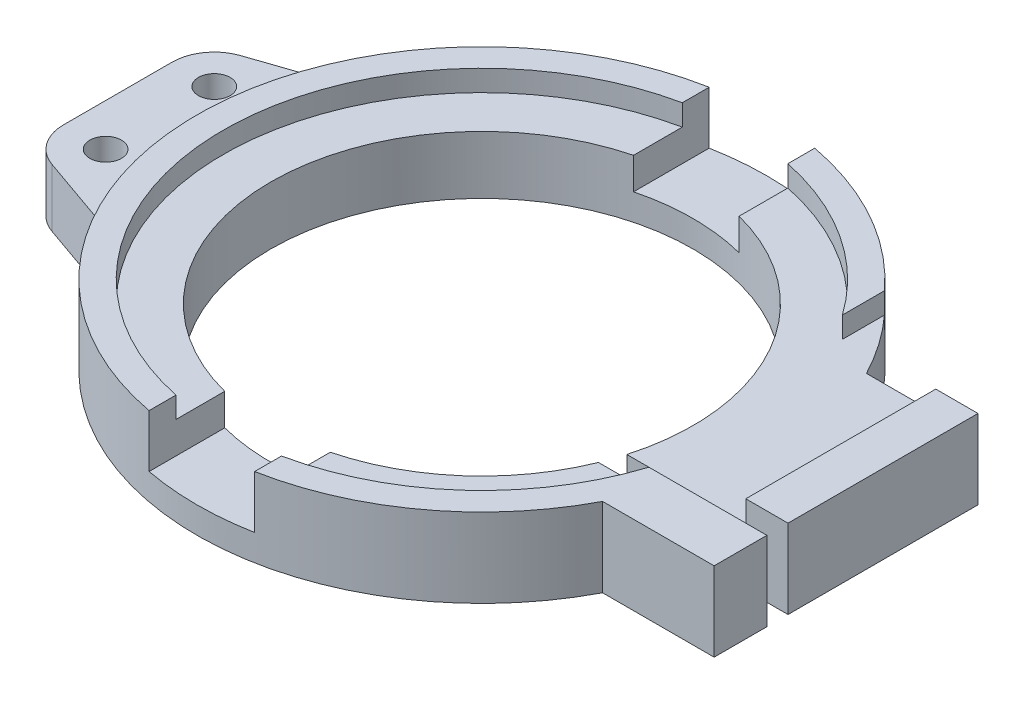
ISO-10303-21;
HEADER;
FILE_DESCRIPTION(('STEP AP214'),'2;1');
FILE_NAME('part.step','',(''),(''),'','','');
FILE_SCHEMA(('AUTOMOTIVE_DESIGN { 1 0 10303 214 1 1 1 1 }'));
ENDSEC;
DATA;
#1=APPLICATION_CONTEXT('core data for automotive mechanical design processes');
#2=APPLICATION_PROTOCOL_DEFINITION('international standard','automotive_design',2000,#1);
#3=PRODUCT_CONTEXT('',#1,'mechanical');
#4=PRODUCT('Part','Part','',(#3));
#5=PRODUCT_RELATED_PRODUCT_CATEGORY('part','',(#4));
#6=PRODUCT_DEFINITION_FORMATION('','',#4);
#7=PRODUCT_DEFINITION_CONTEXT('part definition',#1,'design');
#8=PRODUCT_DEFINITION('design','',#6,#7);
#9=PRODUCT_DEFINITION_SHAPE('','',#8);
#10=(LENGTH_UNIT() NAMED_UNIT(*) SI_UNIT(.MILLI.,.METRE.));
#11=(NAMED_UNIT(*) PLANE_ANGLE_UNIT() SI_UNIT($,.RADIAN.));
#12=(NAMED_UNIT(*) SI_UNIT($,.STERADIAN.) SOLID_ANGLE_UNIT());
#13=UNCERTAINTY_MEASURE_WITH_UNIT(LENGTH_MEASURE(1.E-05),#10,'distance_accuracy_value','');
#14=(GEOMETRIC_REPRESENTATION_CONTEXT(3) GLOBAL_UNCERTAINTY_ASSIGNED_CONTEXT((#13)) GLOBAL_UNIT_ASSIGNED_CONTEXT((#10,
#11,#12)) REPRESENTATION_CONTEXT('',''));
#15=CARTESIAN_POINT('',(0.,0.,0.));
#16=DIRECTION('',(0.,0.,1.));
#17=DIRECTION('',(1.,0.,0.));
#18=AXIS2_PLACEMENT_3D('',#15,#16,#17);
#19=CARTESIAN_POINT('',(0.,15.,0.));
#20=DIRECTION('',(0.,-1.,0.));
#21=DIRECTION('',(0.,0.,-1.));
#22=AXIS2_PLACEMENT_3D('',#19,#20,#21);
#23=CYLINDRICAL_SURFACE('',#22,54.);
#24=DIRECTION('',(0.,-1.,0.));
#25=VECTOR('',#24,1.);
#26=CARTESIAN_POINT('',(47.8643917750973,11.,-25.));
#27=LINE('',#26,#25);
#28=CARTESIAN_POINT('',(47.8643917750973,11.,-25.));
#29=VERTEX_POINT('',#28);
#30=CARTESIAN_POINT('',(47.8643917750973,0.,-25.));
#31=VERTEX_POINT('',#30);
#32=EDGE_CURVE('E58',#29,#31,#27,.T.);
#33=ORIENTED_EDGE('',*,*,#32,.T.);
#34=CARTESIAN_POINT('',(0.,0.,0.));
#35=DIRECTION('',(0.,1.,0.));
#36=DIRECTION('',(0.,0.,1.));
#37=AXIS2_PLACEMENT_3D('',#34,#35,#36);
#38=CIRCLE('',#37,54.);
#39=CARTESIAN_POINT('',(-48.9411888872082,0.,-22.8201671840196));
#40=VERTEX_POINT('',#39);
#41=EDGE_CURVE('E421',#31,#40,#38,.T.);
#42=ORIENTED_EDGE('',*,*,#41,.T.);
#43=DIRECTION('',(0.,-1.,0.));
#44=VECTOR('',#43,1.);
#45=CARTESIAN_POINT('',(-48.9411888872082,11.,-22.8201671840196));
#46=LINE('',#45,#44);
#47=CARTESIAN_POINT('',(-48.9411888872082,11.,-22.8201671840196));
#48=VERTEX_POINT('',#47);
#49=EDGE_CURVE('E414',#48,#40,#46,.T.);
#50=ORIENTED_EDGE('',*,*,#49,.F.);
#51=CARTESIAN_POINT('',(0.,11.,0.));
#52=DIRECTION('',(0.,1.,0.));
#53=DIRECTION('',(0.,0.,1.));
#54=AXIS2_PLACEMENT_3D('',#51,#52,#53);
#55=CIRCLE('',#54,54.);
#56=CARTESIAN_POINT('',(-48.8437412923493,11.,23.0280033126204));
#57=VERTEX_POINT('',#56);
#58=EDGE_CURVE('E379',#48,#57,#55,.T.);
#59=ORIENTED_EDGE('',*,*,#58,.T.);
#60=DIRECTION('',(0.,-1.,0.));
#61=VECTOR('',#60,1.);
#62=CARTESIAN_POINT('',(-48.8437412923493,11.,23.0280033126204));
#63=LINE('',#62,#61);
#64=CARTESIAN_POINT('',(-48.8437412923493,0.,23.0280033126204));
#65=VERTEX_POINT('',#64);
#66=EDGE_CURVE('E420',#57,#65,#63,.T.);
#67=ORIENTED_EDGE('',*,*,#66,.T.);
#68=CARTESIAN_POINT('',(0.,0.,0.));
#69=DIRECTION('',(0.,1.,0.));
#70=DIRECTION('',(0.,0.,1.));
#71=AXIS2_PLACEMENT_3D('',#68,#69,#70);
#72=CIRCLE('',#71,54.);
#73=CARTESIAN_POINT('',(47.8643917750973,0.,25.));
#74=VERTEX_POINT('',#73);
#75=EDGE_CURVE('E456',#65,#74,#72,.T.);
#76=ORIENTED_EDGE('',*,*,#75,.T.);
#77=DIRECTION('',(0.,-1.,0.));
#78=VECTOR('',#77,1.);
#79=CARTESIAN_POINT('',(47.8643917750973,15.,25.));
#80=LINE('',#79,#78);
#81=CARTESIAN_POINT('',(47.8643917750973,15.,25.));
#82=VERTEX_POINT('',#81);
#83=EDGE_CURVE('E491',#82,#74,#80,.T.);
#84=ORIENTED_EDGE('',*,*,#83,.F.);
#85=CARTESIAN_POINT('',(0.,15.,0.));
#86=DIRECTION('',(0.,1.,0.));
#87=DIRECTION('',(0.,0.,1.));
#88=AXIS2_PLACEMENT_3D('',#85,#86,#87);
#89=CIRCLE('',#88,54.);
#90=CARTESIAN_POINT('',(10.,15.,53.0659966456864));
#91=VERTEX_POINT('',#90);
#92=EDGE_CURVE('E467',#91,#82,#89,.T.);
#93=ORIENTED_EDGE('',*,*,#92,.F.);
#94=DIRECTION('',(0.,-1.,0.));
#95=VECTOR('',#94,1.);
#96=CARTESIAN_POINT('',(10.,15.,53.0659966456864));
#97=LINE('',#96,#95);
#98=CARTESIAN_POINT('',(10.,5.,53.0659966456864));
#99=VERTEX_POINT('',#98);
#100=EDGE_CURVE('E492',#91,#99,#97,.T.);
#101=ORIENTED_EDGE('',*,*,#100,.T.);
#102=CARTESIAN_POINT('',(0.,5.,0.));
#103=DIRECTION('',(0.,1.,0.));
#104=DIRECTION('',(0.,0.,1.));
#105=AXIS2_PLACEMENT_3D('',#102,#103,#104);
#106=CIRCLE('',#105,54.);
#107=CARTESIAN_POINT('',(-10.,5.,53.0659966456864));
#108=VERTEX_POINT('',#107);
#109=EDGE_CURVE('E452',#108,#99,#106,.T.);
#110=ORIENTED_EDGE('',*,*,#109,.F.);
#111=DIRECTION('',(0.,-1.,0.));
#112=VECTOR('',#111,1.);
#113=CARTESIAN_POINT('',(-10.,15.,53.0659966456864));
#114=LINE('',#113,#112);
#115=CARTESIAN_POINT('',(-10.,15.,53.0659966456864));
#116=VERTEX_POINT('',#115);
#117=EDGE_CURVE('E436',#116,#108,#114,.T.);
#118=ORIENTED_EDGE('',*,*,#117,.F.);
#119=CARTESIAN_POINT('',(0.,15.,0.));
#120=DIRECTION('',(0.,1.,0.));
#121=DIRECTION('',(0.,0.,1.));
#122=AXIS2_PLACEMENT_3D('',#119,#120,#121);
#123=CIRCLE('',#122,54.);
#124=CARTESIAN_POINT('',(-10.,15.,-53.0659966456864));
#125=VERTEX_POINT('',#124);
#126=EDGE_CURVE('E429',#125,#116,#123,.T.);
#127=ORIENTED_EDGE('',*,*,#126,.F.);
#128=DIRECTION('',(0.,-1.,0.));
#129=VECTOR('',#128,1.);
#130=CARTESIAN_POINT('',(-10.,15.,-53.0659966456864));
#131=LINE('',#130,#129);
#132=CARTESIAN_POINT('',(-10.,5.,-53.0659966456864));
#133=VERTEX_POINT('',#132);
#134=EDGE_CURVE('E437',#125,#133,#131,.T.);
#135=ORIENTED_EDGE('',*,*,#134,.T.);
#136=CARTESIAN_POINT('',(0.,5.,0.));
#137=DIRECTION('',(0.,1.,0.));
#138=DIRECTION('',(0.,0.,1.));
#139=AXIS2_PLACEMENT_3D('',#136,#137,#138);
#140=CIRCLE('',#139,54.);
#141=CARTESIAN_POINT('',(10.,5.,-53.0659966456864));
#142=VERTEX_POINT('',#141);
#143=EDGE_CURVE('E361',#142,#133,#140,.T.);
#144=ORIENTED_EDGE('',*,*,#143,.F.);
#145=DIRECTION('',(0.,-1.,0.));
#146=VECTOR('',#145,1.);
#147=CARTESIAN_POINT('',(10.,15.,-53.0659966456864));
#148=LINE('',#147,#146);
#149=CARTESIAN_POINT('',(10.,15.,-53.0659966456864));
#150=VERTEX_POINT('',#149);
#151=EDGE_CURVE('E349',#150,#142,#148,.T.);
#152=ORIENTED_EDGE('',*,*,#151,.F.);
#153=CARTESIAN_POINT('',(0.,15.,0.));
#154=DIRECTION('',(0.,1.,0.));
#155=DIRECTION('',(0.,0.,1.));
#156=AXIS2_PLACEMENT_3D('',#153,#154,#155);
#157=CIRCLE('',#156,54.);
#158=CARTESIAN_POINT('',(40.,15.,-36.2767142944341));
#159=VERTEX_POINT('',#158);
#160=EDGE_CURVE('E344',#159,#150,#157,.T.);
#161=ORIENTED_EDGE('',*,*,#160,.F.);
#162=DIRECTION('',(0.,-1.,0.));
#163=VECTOR('',#162,1.);
#164=CARTESIAN_POINT('',(40.,15.,-36.2767142944341));
#165=LINE('',#164,#163);
#166=CARTESIAN_POINT('',(40.,11.,-36.2767142944341));
#167=VERTEX_POINT('',#166);
#168=EDGE_CURVE('E355',#159,#167,#165,.T.);
#169=ORIENTED_EDGE('',*,*,#168,.T.);
#170=CARTESIAN_POINT('',(0.,11.,0.));
#171=DIRECTION('',(0.,1.,0.));
#172=DIRECTION('',(0.,0.,1.));
#173=AXIS2_PLACEMENT_3D('',#170,#171,#172);
#174=CIRCLE('',#173,54.);
#175=EDGE_CURVE('E294',#29,#167,#174,.T.);
#176=ORIENTED_EDGE('',*,*,#175,.F.);
#177=EDGE_LOOP('',(#33,#42,#50,#59,#67,#76,#84,#93,#101,#110,#118,#127,#135,#144,#152,#161,#169,#176));
#178=FACE_BOUND('',#177,.T.);
#179=ADVANCED_FACE('F44',(#178),#23,.T.);
#180=CARTESIAN_POINT('',(0.,15.,0.));
#181=DIRECTION('',(0.,-1.,0.));
#182=DIRECTION('',(0.,0.,-1.));
#183=AXIS2_PLACEMENT_3D('',#180,#181,#182);
#184=CYLINDRICAL_SURFACE('',#183,49.);
#185=CARTESIAN_POINT('',(0.,11.,0.));
#186=DIRECTION('',(0.,1.,0.));
#187=DIRECTION('',(0.,0.,1.));
#188=AXIS2_PLACEMENT_3D('',#185,#186,#187);
#189=CIRCLE('',#188,49.);
#190=CARTESIAN_POINT('',(10.,11.,47.9687398208458));
#191=VERTEX_POINT('',#190);
#192=CARTESIAN_POINT('',(46.6476151587624,11.,15.));
#193=VERTEX_POINT('',#192);
#194=EDGE_CURVE('E310',#191,#193,#189,.T.);
#195=ORIENTED_EDGE('',*,*,#194,.F.);
#196=DIRECTION('',(0.,-1.,0.));
#197=VECTOR('',#196,1.);
#198=CARTESIAN_POINT('',(10.,15.,47.9687398208458));
#199=LINE('',#198,#197);
#200=CARTESIAN_POINT('',(10.,15.,47.9687398208458));
#201=VERTEX_POINT('',#200);
#202=EDGE_CURVE('E52',#201,#191,#199,.T.);
#203=ORIENTED_EDGE('',*,*,#202,.F.);
#204=CARTESIAN_POINT('',(0.,15.,0.));
#205=DIRECTION('',(0.,1.,0.));
#206=DIRECTION('',(0.,0.,1.));
#207=AXIS2_PLACEMENT_3D('',#204,#205,#206);
#208=CIRCLE('',#207,49.);
#209=CARTESIAN_POINT('',(46.6476151587624,15.,15.));
#210=VERTEX_POINT('',#209);
#211=EDGE_CURVE('E457',#201,#210,#208,.T.);
#212=ORIENTED_EDGE('',*,*,#211,.T.);
#213=DIRECTION('',(0.,-1.,0.));
#214=VECTOR('',#213,1.);
#215=CARTESIAN_POINT('',(46.6476151587624,15.,15.));
#216=LINE('',#215,#214);
#217=EDGE_CURVE('E476',#210,#193,#216,.T.);
#218=ORIENTED_EDGE('',*,*,#217,.T.);
#219=EDGE_LOOP('',(#195,#203,#212,#218));
#220=FACE_BOUND('',#219,.T.);
#221=ADVANCED_FACE('F50',(#220),#184,.F.);
#222=CARTESIAN_POINT('',(10.,15.,0.));
#223=DIRECTION('',(-1.,0.,0.));
#224=DIRECTION('',(0.,0.,1.));
#225=AXIS2_PLACEMENT_3D('',#222,#223,#224);
#226=PLANE('',#225);
#227=DIRECTION('',(0.,0.,-1.));
#228=VECTOR('',#227,1.);
#229=CARTESIAN_POINT('',(10.,5.,0.));
#230=LINE('',#229,#228);
#231=CARTESIAN_POINT('',(10.,5.,38.7298334620742));
#232=VERTEX_POINT('',#231);
#233=EDGE_CURVE('E451',#99,#232,#230,.T.);
#234=ORIENTED_EDGE('',*,*,#233,.F.);
#235=ORIENTED_EDGE('',*,*,#100,.F.);
#236=DIRECTION('',(0.,0.,-1.));
#237=VECTOR('',#236,1.);
#238=CARTESIAN_POINT('',(10.,15.,0.));
#239=LINE('',#238,#237);
#240=EDGE_CURVE('E464',#91,#201,#239,.T.);
#241=ORIENTED_EDGE('',*,*,#240,.T.);
#242=ORIENTED_EDGE('',*,*,#202,.T.);
#243=DIRECTION('',(0.,0.,-1.));
#244=VECTOR('',#243,1.);
#245=CARTESIAN_POINT('',(10.,11.,0.));
#246=LINE('',#245,#244);
#247=CARTESIAN_POINT('',(10.,11.,38.7298334620742));
#248=VERTEX_POINT('',#247);
#249=EDGE_CURVE('E302',#191,#248,#246,.T.);
#250=ORIENTED_EDGE('',*,*,#249,.T.);
#251=DIRECTION('',(0.,-1.,0.));
#252=VECTOR('',#251,1.);
#253=CARTESIAN_POINT('',(10.,11.,38.7298334620742));
#254=LINE('',#253,#252);
#255=EDGE_CURVE('E314',#248,#232,#254,.T.);
#256=ORIENTED_EDGE('',*,*,#255,.T.);
#257=EDGE_LOOP('',(#234,#235,#241,#242,#250,#256));
#258=FACE_BOUND('',#257,.T.);
#259=ADVANCED_FACE('F497',(#258),#226,.T.);
#260=CARTESIAN_POINT('',(0.,15.,25.));
#261=DIRECTION('',(0.,0.,1.));
#262=DIRECTION('',(1.,0.,0.));
#263=AXIS2_PLACEMENT_3D('',#260,#261,#262);
#264=PLANE('',#263);
#265=DIRECTION('',(-1.,0.,0.));
#266=VECTOR('',#265,1.);
#267=CARTESIAN_POINT('',(0.,0.,25.));
#268=LINE('',#267,#266);
#269=CARTESIAN_POINT('',(69.,0.,25.));
#270=VERTEX_POINT('',#269);
#271=EDGE_CURVE('E477',#270,#74,#268,.T.);
#272=ORIENTED_EDGE('',*,*,#271,.F.);
#273=DIRECTION('',(0.,-1.,0.));
#274=VECTOR('',#273,1.);
#275=CARTESIAN_POINT('',(69.,15.,25.));
#276=LINE('',#275,#274);
#277=CARTESIAN_POINT('',(69.,15.,25.));
#278=VERTEX_POINT('',#277);
#279=EDGE_CURVE('E493',#278,#270,#276,.T.);
#280=ORIENTED_EDGE('',*,*,#279,.F.);
#281=DIRECTION('',(-1.,0.,0.));
#282=VECTOR('',#281,1.);
#283=CARTESIAN_POINT('',(0.,15.,25.));
#284=LINE('',#283,#282);
#285=EDGE_CURVE('E466',#278,#82,#284,.T.);
#286=ORIENTED_EDGE('',*,*,#285,.T.);
#287=ORIENTED_EDGE('',*,*,#83,.T.);
#288=EDGE_LOOP('',(#272,#280,#286,#287));
#289=FACE_BOUND('',#288,.T.);
#290=ADVANCED_FACE('F579',(#289),#264,.T.);
#291=CARTESIAN_POINT('',(69.,15.,0.));
#292=DIRECTION('',(-1.,0.,0.));
#293=DIRECTION('',(0.,0.,1.));
#294=AXIS2_PLACEMENT_3D('',#291,#292,#293);
#295=PLANE('',#294);
#296=DIRECTION('',(0.,0.,-1.));
#297=VECTOR('',#296,1.);
#298=CARTESIAN_POINT('',(69.,0.,0.));
#299=LINE('',#298,#297);
#300=CARTESIAN_POINT('',(69.,0.,15.));
#301=VERTEX_POINT('',#300);
#302=EDGE_CURVE('E484',#270,#301,#299,.T.);
#303=ORIENTED_EDGE('',*,*,#302,.T.);
#304=DIRECTION('',(0.,-1.,0.));
#305=VECTOR('',#304,1.);
#306=CARTESIAN_POINT('',(69.,15.,15.));
#307=LINE('',#306,#305);
#308=CARTESIAN_POINT('',(69.,15.,15.));
#309=VERTEX_POINT('',#308);
#310=EDGE_CURVE('E490',#309,#301,#307,.T.);
#311=ORIENTED_EDGE('',*,*,#310,.F.);
#312=DIRECTION('',(0.,0.,-1.));
#313=VECTOR('',#312,1.);
#314=CARTESIAN_POINT('',(69.,15.,0.));
#315=LINE('',#314,#313);
#316=EDGE_CURVE('E472',#278,#309,#315,.T.);
#317=ORIENTED_EDGE('',*,*,#316,.F.);
#318=ORIENTED_EDGE('',*,*,#279,.T.);
#319=EDGE_LOOP('',(#303,#311,#317,#318));
#320=FACE_BOUND('',#319,.T.);
#321=ADVANCED_FACE('F581',(#320),#295,.F.);
#322=CARTESIAN_POINT('',(0.,15.,15.));
#323=DIRECTION('',(0.,0.,-1.));
#324=DIRECTION('',(-1.,0.,0.));
#325=AXIS2_PLACEMENT_3D('',#322,#323,#324);
#326=PLANE('',#325);
#327=DIRECTION('',(1.,0.,0.));
#328=VECTOR('',#327,1.);
#329=CARTESIAN_POINT('',(0.,0.,15.));
#330=LINE('',#329,#328);
#331=CARTESIAN_POINT('',(37.0809924354783,0.,15.));
#332=VERTEX_POINT('',#331);
#333=EDGE_CURVE('E465',#332,#301,#330,.T.);
#334=ORIENTED_EDGE('',*,*,#333,.F.);
#335=DIRECTION('',(0.,-1.,0.));
#336=VECTOR('',#335,1.);
#337=CARTESIAN_POINT('',(37.0809924354783,11.,15.));
#338=LINE('',#337,#336);
#339=CARTESIAN_POINT('',(37.0809924354783,11.,15.));
#340=VERTEX_POINT('',#339);
#341=EDGE_CURVE('E319',#340,#332,#338,.T.);
#342=ORIENTED_EDGE('',*,*,#341,.F.);
#343=DIRECTION('',(1.,0.,0.));
#344=VECTOR('',#343,1.);
#345=CARTESIAN_POINT('',(0.,11.,15.));
#346=LINE('',#345,#344);
#347=EDGE_CURVE('E307',#340,#193,#346,.T.);
#348=ORIENTED_EDGE('',*,*,#347,.T.);
#349=ORIENTED_EDGE('',*,*,#217,.F.);
#350=DIRECTION('',(1.,0.,0.));
#351=VECTOR('',#350,1.);
#352=CARTESIAN_POINT('',(0.,15.,15.));
#353=LINE('',#352,#351);
#354=EDGE_CURVE('E474',#210,#309,#353,.T.);
#355=ORIENTED_EDGE('',*,*,#354,.T.);
#356=ORIENTED_EDGE('',*,*,#310,.T.);
#357=EDGE_LOOP('',(#334,#342,#348,#349,#355,#356));
#358=FACE_BOUND('',#357,.T.);
#359=ADVANCED_FACE('F515',(#358),#326,.T.);
#360=CARTESIAN_POINT('',(0.,15.,0.));
#361=DIRECTION('',(0.,1.,0.));
#362=DIRECTION('',(0.,0.,1.));
#363=AXIS2_PLACEMENT_3D('',#360,#361,#362);
#364=PLANE('',#363);
#365=ORIENTED_EDGE('',*,*,#211,.F.);
#366=ORIENTED_EDGE('',*,*,#240,.F.);
#367=ORIENTED_EDGE('',*,*,#92,.T.);
#368=ORIENTED_EDGE('',*,*,#285,.F.);
#369=ORIENTED_EDGE('',*,*,#316,.T.);
#370=ORIENTED_EDGE('',*,*,#354,.F.);
#371=EDGE_LOOP('',(#365,#366,#367,#368,#369,#370));
#372=FACE_BOUND('',#371,.T.);
#373=ADVANCED_FACE('F510',(#372),#364,.T.);
#374=CARTESIAN_POINT('',(0.,0.,0.));
#375=DIRECTION('',(0.,1.,0.));
#376=DIRECTION('',(0.,0.,1.));
#377=AXIS2_PLACEMENT_3D('',#374,#375,#376);
#378=PLANE('',#377);
#379=DIRECTION('',(1.,0.,0.));
#380=VECTOR('',#379,1.);
#381=CARTESIAN_POINT('',(0.,0.,11.));
#382=LINE('',#381,#380);
#383=CARTESIAN_POINT('',(38.4577690460588,0.,11.));
#384=VERTEX_POINT('',#383);
#385=CARTESIAN_POINT('',(69.,0.,11.));
#386=VERTEX_POINT('',#385);
#387=EDGE_CURVE('E281',#384,#386,#382,.T.);
#388=ORIENTED_EDGE('',*,*,#387,.F.);
#389=CARTESIAN_POINT('',(0.,0.,0.));
#390=DIRECTION('',(0.,1.,0.));
#391=DIRECTION('',(0.,0.,1.));
#392=AXIS2_PLACEMENT_3D('',#389,#390,#391);
#393=CIRCLE('',#392,40.);
#394=EDGE_CURVE('E444',#384,#332,#393,.T.);
#395=ORIENTED_EDGE('',*,*,#394,.T.);
#396=ORIENTED_EDGE('',*,*,#333,.T.);
#397=ORIENTED_EDGE('',*,*,#302,.F.);
#398=ORIENTED_EDGE('',*,*,#271,.T.);
#399=ORIENTED_EDGE('',*,*,#75,.F.);
#400=DIRECTION('',(0.943781389134908,0.,0.330570248997975));
#401=VECTOR('',#400,1.);
#402=CARTESIAN_POINT('',(-12.5218981177209,0.,35.7501451990038));
#403=LINE('',#402,#401);
#404=CARTESIAN_POINT('',(-63.6445619919838,0.,17.8438462182139));
#405=VERTEX_POINT('',#404);
#406=EDGE_CURVE('E396',#405,#65,#403,.T.);
#407=ORIENTED_EDGE('',*,*,#406,.F.);
#408=CARTESIAN_POINT('',(-61.,0.,10.2935951051346));
#409=DIRECTION('',(0.,1.,0.));
#410=DIRECTION('',(0.,0.,1.));
#411=AXIS2_PLACEMENT_3D('',#408,#409,#410);
#412=CIRCLE('',#411,8.00000000000001);
#413=CARTESIAN_POINT('',(-69.,0.,10.2935951051346));
#414=VERTEX_POINT('',#413);
#415=EDGE_CURVE('E397',#405,#414,#412,.F.);
#416=ORIENTED_EDGE('',*,*,#415,.T.);
#417=DIRECTION('',(0.,0.,-1.));
#418=VECTOR('',#417,1.);
#419=CARTESIAN_POINT('',(-69.,0.,0.));
#420=LINE('',#419,#418);
#421=CARTESIAN_POINT('',(-69.,0.,-10.2935951051346));
#422=VERTEX_POINT('',#421);
#423=EDGE_CURVE('E371',#414,#422,#420,.T.);
#424=ORIENTED_EDGE('',*,*,#423,.T.);
#425=CARTESIAN_POINT('',(-61.,0.,-10.2935951051346));
#426=DIRECTION('',(0.,1.,0.));
#427=DIRECTION('',(0.,0.,1.));
#428=AXIS2_PLACEMENT_3D('',#425,#426,#427);
#429=CIRCLE('',#428,8.00000000000001);
#430=CARTESIAN_POINT('',(-63.5644554510947,0.,-17.8714291122471));
#431=VERTEX_POINT('',#430);
#432=EDGE_CURVE('E403',#431,#422,#429,.T.);
#433=ORIENTED_EDGE('',*,*,#432,.F.);
#434=DIRECTION('',(0.947229250889061,0.,-0.320556931386842));
#435=VECTOR('',#434,1.);
#436=CARTESIAN_POINT('',(-11.9581734753537,0.,-35.3357877930002));
#437=LINE('',#436,#435);
#438=EDGE_CURVE('E405',#431,#40,#437,.T.);
#439=ORIENTED_EDGE('',*,*,#438,.T.);
#440=ORIENTED_EDGE('',*,*,#41,.F.);
#441=DIRECTION('',(-1.,0.,0.));
#442=VECTOR('',#441,1.);
#443=CARTESIAN_POINT('',(0.,0.,-25.));
#444=LINE('',#443,#442);
#445=CARTESIAN_POINT('',(69.,0.,-25.));
#446=VERTEX_POINT('',#445);
#447=EDGE_CURVE('E268',#446,#31,#444,.T.);
#448=ORIENTED_EDGE('',*,*,#447,.F.);
#449=DIRECTION('',(0.,0.,-1.));
#450=VECTOR('',#449,1.);
#451=CARTESIAN_POINT('',(69.,0.,0.));
#452=LINE('',#451,#450);
#453=EDGE_CURVE('E264',#386,#446,#452,.T.);
#454=ORIENTED_EDGE('',*,*,#453,.F.);
#455=EDGE_LOOP('',(#388,#395,#396,#397,#398,#399,#407,#416,#424,#433,#439,#440,#448,#454));
#456=FACE_BOUND('',#455,.T.);
#457=CARTESIAN_POINT('',(-61.,0.,-10.2935951051346));
#458=DIRECTION('',(0.,1.,0.));
#459=DIRECTION('',(0.,0.,1.));
#460=AXIS2_PLACEMENT_3D('',#457,#458,#459);
#461=CIRCLE('',#460,3.);
#462=CARTESIAN_POINT('',(-61.,0.,-7.29359510513458));
#463=VERTEX_POINT('',#462);
#464=EDGE_CURVE('E366',#463,#463,#461,.T.);
#465=ORIENTED_EDGE('',*,*,#464,.T.);
#466=EDGE_LOOP('',(#465));
#467=FACE_BOUND('',#466,.T.);
#468=CARTESIAN_POINT('',(-61.,0.,10.2935951051346));
#469=DIRECTION('',(0.,1.,0.));
#470=DIRECTION('',(0.,0.,1.));
#471=AXIS2_PLACEMENT_3D('',#468,#469,#470);
#472=CIRCLE('',#471,3.);
#473=CARTESIAN_POINT('',(-61.,0.,13.2935951051346));
#474=VERTEX_POINT('',#473);
#475=EDGE_CURVE('E393',#474,#474,#472,.T.);
#476=ORIENTED_EDGE('',*,*,#475,.T.);
#477=EDGE_LOOP('',(#476));
#478=FACE_BOUND('',#477,.T.);
#479=ADVANCED_FACE('F591',(#456,#467,#478),#378,.F.);
#480=CARTESIAN_POINT('',(0.,5.,0.));
#481=DIRECTION('',(0.,-1.,0.));
#482=DIRECTION('',(0.,0.,-1.));
#483=AXIS2_PLACEMENT_3D('',#480,#481,#482);
#484=CYLINDRICAL_SURFACE('',#483,40.);
#485=ORIENTED_EDGE('',*,*,#394,.F.);
#486=DIRECTION('',(0.,-1.,0.));
#487=VECTOR('',#486,1.);
#488=CARTESIAN_POINT('',(38.4577690460588,11.,11.));
#489=LINE('',#488,#487);
#490=CARTESIAN_POINT('',(38.4577690460588,11.,11.));
#491=VERTEX_POINT('',#490);
#492=EDGE_CURVE('E300',#491,#384,#489,.T.);
#493=ORIENTED_EDGE('',*,*,#492,.F.);
#494=CARTESIAN_POINT('',(0.,11.,0.));
#495=DIRECTION('',(0.,1.,0.));
#496=DIRECTION('',(0.,0.,1.));
#497=AXIS2_PLACEMENT_3D('',#494,#495,#496);
#498=CIRCLE('',#497,40.);
#499=CARTESIAN_POINT('',(10.,11.,-38.7298334620742));
#500=VERTEX_POINT('',#499);
#501=EDGE_CURVE('E286',#491,#500,#498,.T.);
#502=ORIENTED_EDGE('',*,*,#501,.T.);
#503=DIRECTION('',(0.,-1.,0.));
#504=VECTOR('',#503,1.);
#505=CARTESIAN_POINT('',(10.,11.,-38.7298334620742));
#506=LINE('',#505,#504);
#507=CARTESIAN_POINT('',(10.,5.,-38.7298334620742));
#508=VERTEX_POINT('',#507);
#509=EDGE_CURVE('E301',#500,#508,#506,.T.);
#510=ORIENTED_EDGE('',*,*,#509,.T.);
#511=CARTESIAN_POINT('',(0.,5.,0.));
#512=DIRECTION('',(0.,1.,0.));
#513=DIRECTION('',(0.,0.,1.));
#514=AXIS2_PLACEMENT_3D('',#511,#512,#513);
#515=CIRCLE('',#514,40.);
#516=CARTESIAN_POINT('',(-10.,5.,-38.7298334620742));
#517=VERTEX_POINT('',#516);
#518=EDGE_CURVE('E356',#508,#517,#515,.T.);
#519=ORIENTED_EDGE('',*,*,#518,.T.);
#520=DIRECTION('',(0.,-1.,0.));
#521=VECTOR('',#520,1.);
#522=CARTESIAN_POINT('',(-10.,11.,-38.7298334620742));
#523=LINE('',#522,#521);
#524=CARTESIAN_POINT('',(-10.,11.,-38.7298334620742));
#525=VERTEX_POINT('',#524);
#526=EDGE_CURVE('E333',#525,#517,#523,.T.);
#527=ORIENTED_EDGE('',*,*,#526,.F.);
#528=CARTESIAN_POINT('',(0.,11.,0.));
#529=DIRECTION('',(0.,1.,0.));
#530=DIRECTION('',(0.,0.,1.));
#531=AXIS2_PLACEMENT_3D('',#528,#529,#530);
#532=CIRCLE('',#531,40.);
#533=CARTESIAN_POINT('',(-10.,11.,38.7298334620742));
#534=VERTEX_POINT('',#533);
#535=EDGE_CURVE('E322',#525,#534,#532,.T.);
#536=ORIENTED_EDGE('',*,*,#535,.T.);
#537=DIRECTION('',(0.,-1.,0.));
#538=VECTOR('',#537,1.);
#539=CARTESIAN_POINT('',(-10.,11.,38.7298334620742));
#540=LINE('',#539,#538);
#541=CARTESIAN_POINT('',(-10.,5.,38.7298334620742));
#542=VERTEX_POINT('',#541);
#543=EDGE_CURVE('E334',#534,#542,#540,.T.);
#544=ORIENTED_EDGE('',*,*,#543,.T.);
#545=CARTESIAN_POINT('',(0.,5.,0.));
#546=DIRECTION('',(0.,1.,0.));
#547=DIRECTION('',(0.,0.,1.));
#548=AXIS2_PLACEMENT_3D('',#545,#546,#547);
#549=CIRCLE('',#548,40.);
#550=EDGE_CURVE('E447',#542,#232,#549,.T.);
#551=ORIENTED_EDGE('',*,*,#550,.T.);
#552=ORIENTED_EDGE('',*,*,#255,.F.);
#553=CARTESIAN_POINT('',(0.,11.,0.));
#554=DIRECTION('',(0.,1.,0.));
#555=DIRECTION('',(0.,0.,1.));
#556=AXIS2_PLACEMENT_3D('',#553,#554,#555);
#557=CIRCLE('',#556,40.);
#558=EDGE_CURVE('E315',#248,#340,#557,.T.);
#559=ORIENTED_EDGE('',*,*,#558,.T.);
#560=ORIENTED_EDGE('',*,*,#341,.T.);
#561=EDGE_LOOP('',(#485,#493,#502,#510,#519,#527,#536,#544,#551,#552,#559,#560));
#562=FACE_BOUND('',#561,.T.);
#563=ADVANCED_FACE('F520',(#562),#484,.F.);
#564=CARTESIAN_POINT('',(0.,5.,0.));
#565=DIRECTION('',(0.,1.,0.));
#566=DIRECTION('',(0.,0.,1.));
#567=AXIS2_PLACEMENT_3D('',#564,#565,#566);
#568=PLANE('',#567);
#569=ORIENTED_EDGE('',*,*,#550,.F.);
#570=DIRECTION('',(0.,0.,-1.));
#571=VECTOR('',#570,1.);
#572=CARTESIAN_POINT('',(-10.,5.,0.));
#573=LINE('',#572,#571);
#574=EDGE_CURVE('E446',#108,#542,#573,.T.);
#575=ORIENTED_EDGE('',*,*,#574,.F.);
#576=ORIENTED_EDGE('',*,*,#109,.T.);
#577=ORIENTED_EDGE('',*,*,#233,.T.);
#578=EDGE_LOOP('',(#569,#575,#576,#577));
#579=FACE_BOUND('',#578,.T.);
#580=ADVANCED_FACE('F524',(#579),#568,.T.);
#581=CARTESIAN_POINT('',(0.,15.,0.));
#582=DIRECTION('',(0.,-1.,0.));
#583=DIRECTION('',(0.,0.,-1.));
#584=AXIS2_PLACEMENT_3D('',#581,#582,#583);
#585=CYLINDRICAL_SURFACE('',#584,49.);
#586=CARTESIAN_POINT('',(0.,11.,0.));
#587=DIRECTION('',(0.,1.,0.));
#588=DIRECTION('',(0.,0.,1.));
#589=AXIS2_PLACEMENT_3D('',#586,#587,#588);
#590=CIRCLE('',#589,49.);
#591=CARTESIAN_POINT('',(-10.,11.,-47.9687398208458));
#592=VERTEX_POINT('',#591);
#593=CARTESIAN_POINT('',(-10.,11.,47.9687398208458));
#594=VERTEX_POINT('',#593);
#595=EDGE_CURVE('E330',#592,#594,#590,.T.);
#596=ORIENTED_EDGE('',*,*,#595,.F.);
#597=DIRECTION('',(0.,-1.,0.));
#598=VECTOR('',#597,1.);
#599=CARTESIAN_POINT('',(-10.,15.,-47.9687398208458));
#600=LINE('',#599,#598);
#601=CARTESIAN_POINT('',(-10.,15.,-47.9687398208458));
#602=VERTEX_POINT('',#601);
#603=EDGE_CURVE('E445',#602,#592,#600,.T.);
#604=ORIENTED_EDGE('',*,*,#603,.F.);
#605=CARTESIAN_POINT('',(0.,15.,0.));
#606=DIRECTION('',(0.,1.,0.));
#607=DIRECTION('',(0.,0.,1.));
#608=AXIS2_PLACEMENT_3D('',#605,#606,#607);
#609=CIRCLE('',#608,49.);
#610=CARTESIAN_POINT('',(-10.,15.,47.9687398208458));
#611=VERTEX_POINT('',#610);
#612=EDGE_CURVE('E425',#602,#611,#609,.T.);
#613=ORIENTED_EDGE('',*,*,#612,.T.);
#614=DIRECTION('',(0.,-1.,0.));
#615=VECTOR('',#614,1.);
#616=CARTESIAN_POINT('',(-10.,15.,47.9687398208458));
#617=LINE('',#616,#615);
#618=EDGE_CURVE('E433',#611,#594,#617,.T.);
#619=ORIENTED_EDGE('',*,*,#618,.T.);
#620=EDGE_LOOP('',(#596,#604,#613,#619));
#621=FACE_BOUND('',#620,.T.);
#622=ADVANCED_FACE('F649',(#621),#585,.F.);
#623=CARTESIAN_POINT('',(-10.,15.,0.));
#624=DIRECTION('',(-1.,0.,0.));
#625=DIRECTION('',(0.,0.,1.));
#626=AXIS2_PLACEMENT_3D('',#623,#624,#625);
#627=PLANE('',#626);
#628=ORIENTED_EDGE('',*,*,#603,.T.);
#629=DIRECTION('',(0.,0.,-1.));
#630=VECTOR('',#629,1.);
#631=CARTESIAN_POINT('',(-10.,11.,0.));
#632=LINE('',#631,#630);
#633=EDGE_CURVE('E321',#525,#592,#632,.T.);
#634=ORIENTED_EDGE('',*,*,#633,.F.);
#635=ORIENTED_EDGE('',*,*,#526,.T.);
#636=DIRECTION('',(0.,0.,-1.));
#637=VECTOR('',#636,1.);
#638=CARTESIAN_POINT('',(-10.,5.,0.));
#639=LINE('',#638,#637);
#640=EDGE_CURVE('E11',#517,#133,#639,.T.);
#641=ORIENTED_EDGE('',*,*,#640,.T.);
#642=ORIENTED_EDGE('',*,*,#134,.F.);
#643=DIRECTION('',(0.,0.,-1.));
#644=VECTOR('',#643,1.);
#645=CARTESIAN_POINT('',(-10.,15.,0.));
#646=LINE('',#645,#644);
#647=EDGE_CURVE('E430',#602,#125,#646,.T.);
#648=ORIENTED_EDGE('',*,*,#647,.F.);
#649=EDGE_LOOP('',(#628,#634,#635,#641,#642,#648));
#650=FACE_BOUND('',#649,.T.);
#651=ADVANCED_FACE('F536',(#650),#627,.F.);
#652=CARTESIAN_POINT('',(-10.,15.,0.));
#653=DIRECTION('',(-1.,0.,0.));
#654=DIRECTION('',(0.,0.,1.));
#655=AXIS2_PLACEMENT_3D('',#652,#653,#654);
#656=PLANE('',#655);
#657=ORIENTED_EDGE('',*,*,#574,.T.);
#658=ORIENTED_EDGE('',*,*,#543,.F.);
#659=DIRECTION('',(0.,0.,-1.));
#660=VECTOR('',#659,1.);
#661=CARTESIAN_POINT('',(-10.,11.,0.));
#662=LINE('',#661,#660);
#663=EDGE_CURVE('E329',#594,#534,#662,.T.);
#664=ORIENTED_EDGE('',*,*,#663,.F.);
#665=ORIENTED_EDGE('',*,*,#618,.F.);
#666=DIRECTION('',(0.,0.,-1.));
#667=VECTOR('',#666,1.);
#668=CARTESIAN_POINT('',(-10.,15.,0.));
#669=LINE('',#668,#667);
#670=EDGE_CURVE('E431',#116,#611,#669,.T.);
#671=ORIENTED_EDGE('',*,*,#670,.F.);
#672=ORIENTED_EDGE('',*,*,#117,.T.);
#673=EDGE_LOOP('',(#657,#658,#664,#665,#671,#672));
#674=FACE_BOUND('',#673,.T.);
#675=ADVANCED_FACE('F526',(#674),#656,.F.);
#676=CARTESIAN_POINT('',(0.,15.,0.));
#677=DIRECTION('',(0.,1.,0.));
#678=DIRECTION('',(0.,0.,1.));
#679=AXIS2_PLACEMENT_3D('',#676,#677,#678);
#680=PLANE('',#679);
#681=ORIENTED_EDGE('',*,*,#612,.F.);
#682=ORIENTED_EDGE('',*,*,#647,.T.);
#683=ORIENTED_EDGE('',*,*,#126,.T.);
#684=ORIENTED_EDGE('',*,*,#670,.T.);
#685=EDGE_LOOP('',(#681,#682,#683,#684));
#686=FACE_BOUND('',#685,.T.);
#687=ADVANCED_FACE('F537',(#686),#680,.T.);
#688=CARTESIAN_POINT('',(-61.,11.,10.2935951051346));
#689=DIRECTION('',(0.,-1.,0.));
#690=DIRECTION('',(0.,0.,-1.));
#691=AXIS2_PLACEMENT_3D('',#688,#689,#690);
#692=CYLINDRICAL_SURFACE('',#691,8.00000000000001);
#693=ORIENTED_EDGE('',*,*,#415,.F.);
#694=DIRECTION('',(0.,-1.,0.));
#695=VECTOR('',#694,1.);
#696=CARTESIAN_POINT('',(-63.6445619919838,11.,17.8438462182139));
#697=LINE('',#696,#695);
#698=CARTESIAN_POINT('',(-63.6445619919838,11.,17.8438462182139));
#699=VERTEX_POINT('',#698);
#700=EDGE_CURVE('E423',#699,#405,#697,.T.);
#701=ORIENTED_EDGE('',*,*,#700,.F.);
#702=CARTESIAN_POINT('',(-61.,11.,10.2935951051346));
#703=DIRECTION('',(0.,1.,0.));
#704=DIRECTION('',(0.,0.,1.));
#705=AXIS2_PLACEMENT_3D('',#702,#703,#704);
#706=CIRCLE('',#705,8.00000000000001);
#707=CARTESIAN_POINT('',(-69.,11.,10.2935951051346));
#708=VERTEX_POINT('',#707);
#709=EDGE_CURVE('E372',#699,#708,#706,.F.);
#710=ORIENTED_EDGE('',*,*,#709,.T.);
#711=DIRECTION('',(0.,-1.,0.));
#712=VECTOR('',#711,1.);
#713=CARTESIAN_POINT('',(-69.,11.,10.2935951051346));
#714=LINE('',#713,#712);
#715=EDGE_CURVE('E388',#708,#414,#714,.T.);
#716=ORIENTED_EDGE('',*,*,#715,.T.);
#717=EDGE_LOOP('',(#693,#701,#710,#716));
#718=FACE_BOUND('',#717,.T.);
#719=ADVANCED_FACE('F603',(#718),#692,.T.);
#720=CARTESIAN_POINT('',(-12.5218981177209,11.,35.7501451990038));
#721=DIRECTION('',(0.330570248997975,0.,-0.943781389134908));
#722=DIRECTION('',(-0.943781389134908,0.,-0.330570248997975));
#723=AXIS2_PLACEMENT_3D('',#720,#721,#722);
#724=PLANE('',#723);
#725=ORIENTED_EDGE('',*,*,#406,.T.);
#726=ORIENTED_EDGE('',*,*,#66,.F.);
#727=DIRECTION('',(0.943781389134908,0.,0.330570248997975));
#728=VECTOR('',#727,1.);
#729=CARTESIAN_POINT('',(-12.5218981177209,11.,35.7501451990038));
#730=LINE('',#729,#728);
#731=EDGE_CURVE('E380',#699,#57,#730,.T.);
#732=ORIENTED_EDGE('',*,*,#731,.F.);
#733=ORIENTED_EDGE('',*,*,#700,.T.);
#734=EDGE_LOOP('',(#725,#726,#732,#733));
#735=FACE_BOUND('',#734,.T.);
#736=ADVANCED_FACE('F602',(#735),#724,.F.);
#737=CARTESIAN_POINT('',(-11.9581734753537,11.,-35.3357877930002));
#738=DIRECTION('',(-0.320556931386842,0.,-0.947229250889061));
#739=DIRECTION('',(-0.947229250889061,0.,0.320556931386842));
#740=AXIS2_PLACEMENT_3D('',#737,#738,#739);
#741=PLANE('',#740);
#742=ORIENTED_EDGE('',*,*,#438,.F.);
#743=DIRECTION('',(0.,-1.,0.));
#744=VECTOR('',#743,1.);
#745=CARTESIAN_POINT('',(-63.5644554510947,11.,-17.8714291122471));
#746=LINE('',#745,#744);
#747=CARTESIAN_POINT('',(-63.5644554510947,11.,-17.8714291122471));
#748=VERTEX_POINT('',#747);
#749=EDGE_CURVE('E413',#748,#431,#746,.T.);
#750=ORIENTED_EDGE('',*,*,#749,.F.);
#751=DIRECTION('',(0.947229250889061,0.,-0.320556931386842));
#752=VECTOR('',#751,1.);
#753=CARTESIAN_POINT('',(-11.9581734753537,11.,-35.3357877930002));
#754=LINE('',#753,#752);
#755=EDGE_CURVE('E385',#748,#48,#754,.T.);
#756=ORIENTED_EDGE('',*,*,#755,.T.);
#757=ORIENTED_EDGE('',*,*,#49,.T.);
#758=EDGE_LOOP('',(#742,#750,#756,#757));
#759=FACE_BOUND('',#758,.T.);
#760=ADVANCED_FACE('F618',(#759),#741,.T.);
#761=CARTESIAN_POINT('',(-61.,11.,-10.2935951051346));
#762=DIRECTION('',(0.,-1.,0.));
#763=DIRECTION('',(0.,0.,-1.));
#764=AXIS2_PLACEMENT_3D('',#761,#762,#763);
#765=CYLINDRICAL_SURFACE('',#764,8.00000000000001);
#766=ORIENTED_EDGE('',*,*,#432,.T.);
#767=DIRECTION('',(0.,-1.,0.));
#768=VECTOR('',#767,1.);
#769=CARTESIAN_POINT('',(-69.,11.,-10.2935951051346));
#770=LINE('',#769,#768);
#771=CARTESIAN_POINT('',(-69.,11.,-10.2935951051346));
#772=VERTEX_POINT('',#771);
#773=EDGE_CURVE('E411',#772,#422,#770,.T.);
#774=ORIENTED_EDGE('',*,*,#773,.F.);
#775=CARTESIAN_POINT('',(-61.,11.,-10.2935951051346));
#776=DIRECTION('',(0.,1.,0.));
#777=DIRECTION('',(0.,0.,1.));
#778=AXIS2_PLACEMENT_3D('',#775,#776,#777);
#779=CIRCLE('',#778,8.00000000000001);
#780=EDGE_CURVE('E383',#748,#772,#779,.T.);
#781=ORIENTED_EDGE('',*,*,#780,.F.);
#782=ORIENTED_EDGE('',*,*,#749,.T.);
#783=EDGE_LOOP('',(#766,#774,#781,#782));
#784=FACE_BOUND('',#783,.T.);
#785=ADVANCED_FACE('F619',(#784),#765,.T.);
#786=CARTESIAN_POINT('',(-61.,11.,10.2935951051346));
#787=DIRECTION('',(0.,-1.,0.));
#788=DIRECTION('',(0.,0.,-1.));
#789=AXIS2_PLACEMENT_3D('',#786,#787,#788);
#790=CYLINDRICAL_SURFACE('',#789,3.);
#791=CARTESIAN_POINT('',(-61.,11.,10.2935951051346));
#792=DIRECTION('',(0.,1.,0.));
#793=DIRECTION('',(0.,0.,1.));
#794=AXIS2_PLACEMENT_3D('',#791,#792,#793);
#795=CIRCLE('',#794,3.);
#796=CARTESIAN_POINT('',(-61.,11.,13.2935951051346));
#797=VERTEX_POINT('',#796);
#798=EDGE_CURVE('E369',#797,#797,#795,.T.);
#799=ORIENTED_EDGE('',*,*,#798,.T.);
#800=EDGE_LOOP('',(#799));
#801=FACE_BOUND('',#800,.T.);
#802=ORIENTED_EDGE('',*,*,#475,.F.);
#803=EDGE_LOOP('',(#802));
#804=FACE_BOUND('',#803,.T.);
#805=ADVANCED_FACE('F625',(#801,#804),#790,.F.);
#806=CARTESIAN_POINT('',(-61.,11.,-10.2935951051346));
#807=DIRECTION('',(0.,-1.,0.));
#808=DIRECTION('',(0.,0.,-1.));
#809=AXIS2_PLACEMENT_3D('',#806,#807,#808);
#810=CYLINDRICAL_SURFACE('',#809,3.);
#811=CARTESIAN_POINT('',(-61.,11.,-10.2935951051346));
#812=DIRECTION('',(0.,1.,0.));
#813=DIRECTION('',(0.,0.,1.));
#814=AXIS2_PLACEMENT_3D('',#811,#812,#813);
#815=CIRCLE('',#814,3.);
#816=CARTESIAN_POINT('',(-61.,11.,-7.29359510513458));
#817=VERTEX_POINT('',#816);
#818=EDGE_CURVE('E370',#817,#817,#815,.T.);
#819=ORIENTED_EDGE('',*,*,#818,.T.);
#820=EDGE_LOOP('',(#819));
#821=FACE_BOUND('',#820,.T.);
#822=ORIENTED_EDGE('',*,*,#464,.F.);
#823=EDGE_LOOP('',(#822));
#824=FACE_BOUND('',#823,.T.);
#825=ADVANCED_FACE('F628',(#821,#824),#810,.F.);
#826=CARTESIAN_POINT('',(-69.,11.,0.));
#827=DIRECTION('',(-1.,0.,0.));
#828=DIRECTION('',(0.,0.,1.));
#829=AXIS2_PLACEMENT_3D('',#826,#827,#828);
#830=PLANE('',#829);
#831=ORIENTED_EDGE('',*,*,#423,.F.);
#832=ORIENTED_EDGE('',*,*,#715,.F.);
#833=DIRECTION('',(0.,0.,-1.));
#834=VECTOR('',#833,1.);
#835=CARTESIAN_POINT('',(-69.,11.,0.));
#836=LINE('',#835,#834);
#837=EDGE_CURVE('E390',#708,#772,#836,.T.);
#838=ORIENTED_EDGE('',*,*,#837,.T.);
#839=ORIENTED_EDGE('',*,*,#773,.T.);
#840=EDGE_LOOP('',(#831,#832,#838,#839));
#841=FACE_BOUND('',#840,.T.);
#842=ADVANCED_FACE('F607',(#841),#830,.T.);
#843=CARTESIAN_POINT('',(0.,11.,0.));
#844=DIRECTION('',(0.,1.,0.));
#845=DIRECTION('',(0.,0.,1.));
#846=AXIS2_PLACEMENT_3D('',#843,#844,#845);
#847=PLANE('',#846);
#848=ORIENTED_EDGE('',*,*,#818,.F.);
#849=EDGE_LOOP('',(#848));
#850=FACE_BOUND('',#849,.T.);
#851=ORIENTED_EDGE('',*,*,#798,.F.);
#852=EDGE_LOOP('',(#851));
#853=FACE_BOUND('',#852,.T.);
#854=ORIENTED_EDGE('',*,*,#709,.F.);
#855=ORIENTED_EDGE('',*,*,#731,.T.);
#856=ORIENTED_EDGE('',*,*,#58,.F.);
#857=ORIENTED_EDGE('',*,*,#755,.F.);
#858=ORIENTED_EDGE('',*,*,#780,.T.);
#859=ORIENTED_EDGE('',*,*,#837,.F.);
#860=EDGE_LOOP('',(#854,#855,#856,#857,#858,#859));
#861=FACE_BOUND('',#860,.T.);
#862=ADVANCED_FACE('F569',(#850,#853,#861),#847,.T.);
#863=CARTESIAN_POINT('',(0.,5.,0.));
#864=DIRECTION('',(0.,1.,0.));
#865=DIRECTION('',(0.,0.,1.));
#866=AXIS2_PLACEMENT_3D('',#863,#864,#865);
#867=PLANE('',#866);
#868=ORIENTED_EDGE('',*,*,#518,.F.);
#869=DIRECTION('',(0.,0.,-1.));
#870=VECTOR('',#869,1.);
#871=CARTESIAN_POINT('',(10.,5.,0.));
#872=LINE('',#871,#870);
#873=EDGE_CURVE('E363',#508,#142,#872,.T.);
#874=ORIENTED_EDGE('',*,*,#873,.T.);
#875=ORIENTED_EDGE('',*,*,#143,.T.);
#876=ORIENTED_EDGE('',*,*,#640,.F.);
#877=EDGE_LOOP('',(#868,#874,#875,#876));
#878=FACE_BOUND('',#877,.T.);
#879=ADVANCED_FACE('F545',(#878),#867,.T.);
#880=CARTESIAN_POINT('',(0.,15.,0.));
#881=DIRECTION('',(0.,-1.,0.));
#882=DIRECTION('',(0.,0.,-1.));
#883=AXIS2_PLACEMENT_3D('',#880,#881,#882);
#884=CYLINDRICAL_SURFACE('',#883,49.);
#885=CARTESIAN_POINT('',(0.,11.,0.));
#886=DIRECTION('',(0.,1.,0.));
#887=DIRECTION('',(0.,0.,1.));
#888=AXIS2_PLACEMENT_3D('',#885,#886,#887);
#889=CIRCLE('',#888,49.);
#890=CARTESIAN_POINT('',(40.,11.,-28.3019433961698));
#891=VERTEX_POINT('',#890);
#892=CARTESIAN_POINT('',(10.,11.,-47.9687398208458));
#893=VERTEX_POINT('',#892);
#894=EDGE_CURVE('E68',#891,#893,#889,.T.);
#895=ORIENTED_EDGE('',*,*,#894,.F.);
#896=DIRECTION('',(0.,-1.,0.));
#897=VECTOR('',#896,1.);
#898=CARTESIAN_POINT('',(40.,15.,-28.3019433961698));
#899=LINE('',#898,#897);
#900=CARTESIAN_POINT('',(40.,15.,-28.3019433961698));
#901=VERTEX_POINT('',#900);
#902=EDGE_CURVE('E358',#901,#891,#899,.T.);
#903=ORIENTED_EDGE('',*,*,#902,.F.);
#904=CARTESIAN_POINT('',(0.,15.,0.));
#905=DIRECTION('',(0.,1.,0.));
#906=DIRECTION('',(0.,0.,1.));
#907=AXIS2_PLACEMENT_3D('',#904,#905,#906);
#908=CIRCLE('',#907,49.);
#909=CARTESIAN_POINT('',(10.,15.,-47.9687398208458));
#910=VERTEX_POINT('',#909);
#911=EDGE_CURVE('E336',#901,#910,#908,.T.);
#912=ORIENTED_EDGE('',*,*,#911,.T.);
#913=DIRECTION('',(0.,-1.,0.));
#914=VECTOR('',#913,1.);
#915=CARTESIAN_POINT('',(10.,15.,-47.9687398208458));
#916=LINE('',#915,#914);
#917=EDGE_CURVE('E348',#910,#893,#916,.T.);
#918=ORIENTED_EDGE('',*,*,#917,.T.);
#919=EDGE_LOOP('',(#895,#903,#912,#918));
#920=FACE_BOUND('',#919,.T.);
#921=ADVANCED_FACE('F565',(#920),#884,.F.);
#922=CARTESIAN_POINT('',(40.,15.,0.));
#923=DIRECTION('',(-1.,0.,0.));
#924=DIRECTION('',(0.,0.,1.));
#925=AXIS2_PLACEMENT_3D('',#922,#923,#924);
#926=PLANE('',#925);
#927=ORIENTED_EDGE('',*,*,#902,.T.);
#928=DIRECTION('',(0.,0.,-1.));
#929=VECTOR('',#928,1.);
#930=CARTESIAN_POINT('',(40.,11.,0.));
#931=LINE('',#930,#929);
#932=EDGE_CURVE('E285',#891,#167,#931,.T.);
#933=ORIENTED_EDGE('',*,*,#932,.T.);
#934=ORIENTED_EDGE('',*,*,#168,.F.);
#935=DIRECTION('',(0.,0.,-1.));
#936=VECTOR('',#935,1.);
#937=CARTESIAN_POINT('',(40.,15.,0.));
#938=LINE('',#937,#936);
#939=EDGE_CURVE('E342',#901,#159,#938,.T.);
#940=ORIENTED_EDGE('',*,*,#939,.F.);
#941=EDGE_LOOP('',(#927,#933,#934,#940));
#942=FACE_BOUND('',#941,.T.);
#943=ADVANCED_FACE('F555',(#942),#926,.F.);
#944=CARTESIAN_POINT('',(10.,15.,0.));
#945=DIRECTION('',(-1.,0.,0.));
#946=DIRECTION('',(0.,0.,1.));
#947=AXIS2_PLACEMENT_3D('',#944,#945,#946);
#948=PLANE('',#947);
#949=ORIENTED_EDGE('',*,*,#151,.T.);
#950=ORIENTED_EDGE('',*,*,#873,.F.);
#951=ORIENTED_EDGE('',*,*,#509,.F.);
#952=DIRECTION('',(0.,0.,-1.));
#953=VECTOR('',#952,1.);
#954=CARTESIAN_POINT('',(10.,11.,0.));
#955=LINE('',#954,#953);
#956=EDGE_CURVE('E287',#500,#893,#955,.T.);
#957=ORIENTED_EDGE('',*,*,#956,.T.);
#958=ORIENTED_EDGE('',*,*,#917,.F.);
#959=DIRECTION('',(0.,0.,-1.));
#960=VECTOR('',#959,1.);
#961=CARTESIAN_POINT('',(10.,15.,0.));
#962=LINE('',#961,#960);
#963=EDGE_CURVE('E343',#910,#150,#962,.T.);
#964=ORIENTED_EDGE('',*,*,#963,.T.);
#965=EDGE_LOOP('',(#949,#950,#951,#957,#958,#964));
#966=FACE_BOUND('',#965,.T.);
#967=ADVANCED_FACE('F549',(#966),#948,.T.);
#968=CARTESIAN_POINT('',(0.,15.,0.));
#969=DIRECTION('',(0.,1.,0.));
#970=DIRECTION('',(0.,0.,1.));
#971=AXIS2_PLACEMENT_3D('',#968,#969,#970);
#972=PLANE('',#971);
#973=ORIENTED_EDGE('',*,*,#911,.F.);
#974=ORIENTED_EDGE('',*,*,#939,.T.);
#975=ORIENTED_EDGE('',*,*,#160,.T.);
#976=ORIENTED_EDGE('',*,*,#963,.F.);
#977=EDGE_LOOP('',(#973,#974,#975,#976));
#978=FACE_BOUND('',#977,.T.);
#979=ADVANCED_FACE('F561',(#978),#972,.T.);
#980=CARTESIAN_POINT('',(0.,11.,0.));
#981=DIRECTION('',(0.,1.,0.));
#982=DIRECTION('',(0.,0.,1.));
#983=AXIS2_PLACEMENT_3D('',#980,#981,#982);
#984=PLANE('',#983);
#985=ORIENTED_EDGE('',*,*,#535,.F.);
#986=ORIENTED_EDGE('',*,*,#633,.T.);
#987=ORIENTED_EDGE('',*,*,#595,.T.);
#988=ORIENTED_EDGE('',*,*,#663,.T.);
#989=EDGE_LOOP('',(#985,#986,#987,#988));
#990=FACE_BOUND('',#989,.T.);
#991=ADVANCED_FACE('F771',(#990),#984,.T.);
#992=CARTESIAN_POINT('',(0.,11.,0.));
#993=DIRECTION('',(0.,1.,0.));
#994=DIRECTION('',(0.,0.,1.));
#995=AXIS2_PLACEMENT_3D('',#992,#993,#994);
#996=PLANE('',#995);
#997=ORIENTED_EDGE('',*,*,#249,.F.);
#998=ORIENTED_EDGE('',*,*,#194,.T.);
#999=ORIENTED_EDGE('',*,*,#347,.F.);
#1000=ORIENTED_EDGE('',*,*,#558,.F.);
#1001=EDGE_LOOP('',(#997,#998,#999,#1000));
#1002=FACE_BOUND('',#1001,.T.);
#1003=ADVANCED_FACE('F513',(#1002),#996,.T.);
#1004=CARTESIAN_POINT('',(0.,11.,11.));
#1005=DIRECTION('',(0.,0.,-1.));
#1006=DIRECTION('',(-1.,0.,0.));
#1007=AXIS2_PLACEMENT_3D('',#1004,#1005,#1006);
#1008=PLANE('',#1007);
#1009=ORIENTED_EDGE('',*,*,#387,.T.);
#1010=DIRECTION('',(0.,-1.,0.));
#1011=VECTOR('',#1010,1.);
#1012=CARTESIAN_POINT('',(69.,15.,11.));
#1013=LINE('',#1012,#1011);
#1014=CARTESIAN_POINT('',(69.,15.,11.));
#1015=VERTEX_POINT('',#1014);
#1016=EDGE_CURVE('E274',#1015,#386,#1013,.T.);
#1017=ORIENTED_EDGE('',*,*,#1016,.F.);
#1018=DIRECTION('',(1.,0.,0.));
#1019=VECTOR('',#1018,1.);
#1020=CARTESIAN_POINT('',(0.,15.,11.));
#1021=LINE('',#1020,#1019);
#1022=CARTESIAN_POINT('',(61.,15.,11.));
#1023=VERTEX_POINT('',#1022);
#1024=EDGE_CURVE('E257',#1023,#1015,#1021,.T.);
#1025=ORIENTED_EDGE('',*,*,#1024,.F.);
#1026=DIRECTION('',(0.,-1.,0.));
#1027=VECTOR('',#1026,1.);
#1028=CARTESIAN_POINT('',(61.,15.,11.));
#1029=LINE('',#1028,#1027);
#1030=CARTESIAN_POINT('',(61.,11.,11.));
#1031=VERTEX_POINT('',#1030);
#1032=EDGE_CURVE('E254',#1023,#1031,#1029,.T.);
#1033=ORIENTED_EDGE('',*,*,#1032,.T.);
#1034=DIRECTION('',(1.,0.,0.));
#1035=VECTOR('',#1034,1.);
#1036=CARTESIAN_POINT('',(0.,11.,11.));
#1037=LINE('',#1036,#1035);
#1038=EDGE_CURVE('E292',#491,#1031,#1037,.T.);
#1039=ORIENTED_EDGE('',*,*,#1038,.F.);
#1040=ORIENTED_EDGE('',*,*,#492,.T.);
#1041=EDGE_LOOP('',(#1009,#1017,#1025,#1033,#1039,#1040));
#1042=FACE_BOUND('',#1041,.T.);
#1043=ADVANCED_FACE('F791',(#1042),#1008,.F.);
#1044=CARTESIAN_POINT('',(0.,11.,0.));
#1045=DIRECTION('',(0.,1.,0.));
#1046=DIRECTION('',(0.,0.,1.));
#1047=AXIS2_PLACEMENT_3D('',#1044,#1045,#1046);
#1048=PLANE('',#1047);
#1049=ORIENTED_EDGE('',*,*,#932,.F.);
#1050=ORIENTED_EDGE('',*,*,#894,.T.);
#1051=ORIENTED_EDGE('',*,*,#956,.F.);
#1052=ORIENTED_EDGE('',*,*,#501,.F.);
#1053=ORIENTED_EDGE('',*,*,#1038,.T.);
#1054=DIRECTION('',(0.,0.,1.));
#1055=VECTOR('',#1054,1.);
#1056=CARTESIAN_POINT('',(61.,11.,0.));
#1057=LINE('',#1056,#1055);
#1058=CARTESIAN_POINT('',(61.,11.,-25.));
#1059=VERTEX_POINT('',#1058);
#1060=EDGE_CURVE('E275',#1059,#1031,#1057,.T.);
#1061=ORIENTED_EDGE('',*,*,#1060,.F.);
#1062=DIRECTION('',(-1.,0.,0.));
#1063=VECTOR('',#1062,1.);
#1064=CARTESIAN_POINT('',(0.,11.,-25.));
#1065=LINE('',#1064,#1063);
#1066=EDGE_CURVE('E270',#1059,#29,#1065,.T.);
#1067=ORIENTED_EDGE('',*,*,#1066,.T.);
#1068=ORIENTED_EDGE('',*,*,#175,.T.);
#1069=EDGE_LOOP('',(#1049,#1050,#1051,#1052,#1053,#1061,#1067,#1068));
#1070=FACE_BOUND('',#1069,.T.);
#1071=ADVANCED_FACE('F548',(#1070),#1048,.T.);
#1072=CARTESIAN_POINT('',(0.,11.,-25.));
#1073=DIRECTION('',(0.,0.,1.));
#1074=DIRECTION('',(1.,0.,0.));
#1075=AXIS2_PLACEMENT_3D('',#1072,#1073,#1074);
#1076=PLANE('',#1075);
#1077=ORIENTED_EDGE('',*,*,#447,.T.);
#1078=ORIENTED_EDGE('',*,*,#32,.F.);
#1079=ORIENTED_EDGE('',*,*,#1066,.F.);
#1080=DIRECTION('',(0.,-1.,0.));
#1081=VECTOR('',#1080,1.);
#1082=CARTESIAN_POINT('',(61.,15.,-25.));
#1083=LINE('',#1082,#1081);
#1084=CARTESIAN_POINT('',(61.,15.,-25.));
#1085=VERTEX_POINT('',#1084);
#1086=EDGE_CURVE('E252',#1085,#1059,#1083,.T.);
#1087=ORIENTED_EDGE('',*,*,#1086,.F.);
#1088=DIRECTION('',(-1.,0.,0.));
#1089=VECTOR('',#1088,1.);
#1090=CARTESIAN_POINT('',(0.,15.,-25.));
#1091=LINE('',#1090,#1089);
#1092=CARTESIAN_POINT('',(69.,15.,-25.));
#1093=VERTEX_POINT('',#1092);
#1094=EDGE_CURVE('E260',#1093,#1085,#1091,.T.);
#1095=ORIENTED_EDGE('',*,*,#1094,.F.);
#1096=DIRECTION('',(0.,-1.,0.));
#1097=VECTOR('',#1096,1.);
#1098=CARTESIAN_POINT('',(69.,15.,-25.));
#1099=LINE('',#1098,#1097);
#1100=EDGE_CURVE('E1163',#1093,#446,#1099,.T.);
#1101=ORIENTED_EDGE('',*,*,#1100,.T.);
#1102=EDGE_LOOP('',(#1077,#1078,#1079,#1087,#1095,#1101));
#1103=FACE_BOUND('',#1102,.T.);
#1104=ADVANCED_FACE('F269',(#1103),#1076,.F.);
#1105=CARTESIAN_POINT('',(61.,15.,0.));
#1106=DIRECTION('',(1.,0.,0.));
#1107=DIRECTION('',(0.,0.,-1.));
#1108=AXIS2_PLACEMENT_3D('',#1105,#1106,#1107);
#1109=PLANE('',#1108);
#1110=ORIENTED_EDGE('',*,*,#1060,.T.);
#1111=ORIENTED_EDGE('',*,*,#1032,.F.);
#1112=DIRECTION('',(0.,0.,1.));
#1113=VECTOR('',#1112,1.);
#1114=CARTESIAN_POINT('',(61.,15.,0.));
#1115=LINE('',#1114,#1113);
#1116=EDGE_CURVE('E250',#1085,#1023,#1115,.T.);
#1117=ORIENTED_EDGE('',*,*,#1116,.F.);
#1118=ORIENTED_EDGE('',*,*,#1086,.T.);
#1119=EDGE_LOOP('',(#1110,#1111,#1117,#1118));
#1120=FACE_BOUND('',#1119,.T.);
#1121=ADVANCED_FACE('F248',(#1120),#1109,.F.);
#1122=CARTESIAN_POINT('',(69.,15.,0.));
#1123=DIRECTION('',(-1.,0.,0.));
#1124=DIRECTION('',(0.,0.,1.));
#1125=AXIS2_PLACEMENT_3D('',#1122,#1123,#1124);
#1126=PLANE('',#1125);
#1127=ORIENTED_EDGE('',*,*,#453,.T.);
#1128=ORIENTED_EDGE('',*,*,#1100,.F.);
#1129=DIRECTION('',(0.,0.,-1.));
#1130=VECTOR('',#1129,1.);
#1131=CARTESIAN_POINT('',(69.,15.,0.));
#1132=LINE('',#1131,#1130);
#1133=EDGE_CURVE('E265',#1015,#1093,#1132,.T.);
#1134=ORIENTED_EDGE('',*,*,#1133,.F.);
#1135=ORIENTED_EDGE('',*,*,#1016,.T.);
#1136=EDGE_LOOP('',(#1127,#1128,#1134,#1135));
#1137=FACE_BOUND('',#1136,.T.);
#1138=ADVANCED_FACE('F830',(#1137),#1126,.F.);
#1139=CARTESIAN_POINT('',(0.,15.,0.));
#1140=DIRECTION('',(0.,1.,0.));
#1141=DIRECTION('',(0.,0.,1.));
#1142=AXIS2_PLACEMENT_3D('',#1139,#1140,#1141);
#1143=PLANE('',#1142);
#1144=ORIENTED_EDGE('',*,*,#1094,.T.);
#1145=ORIENTED_EDGE('',*,*,#1116,.T.);
#1146=ORIENTED_EDGE('',*,*,#1024,.T.);
#1147=ORIENTED_EDGE('',*,*,#1133,.T.);
#1148=EDGE_LOOP('',(#1144,#1145,#1146,#1147));
#1149=FACE_BOUND('',#1148,.T.);
#1150=ADVANCED_FACE('F258',(#1149),#1143,.T.);
#1151=CLOSED_SHELL('',(#179,#221,#259,#290,#321,#359,#373,#479,#563,#580,#622,#651,#675,#687,
#719,#736,#760,#785,#805,#825,#842,#862,#879,#921,#943,#967,#979,#991,#1003,#1043,#1071,#1104,
#1121,#1138,#1150));
#1152=MANIFOLD_SOLID_BREP('B2',#1151);
#1153=ADVANCED_BREP_SHAPE_REPRESENTATION('',(#18,#1152),#14);
#1154=SHAPE_DEFINITION_REPRESENTATION(#9,#1153);
ENDSEC;
END-ISO-10303-21;
